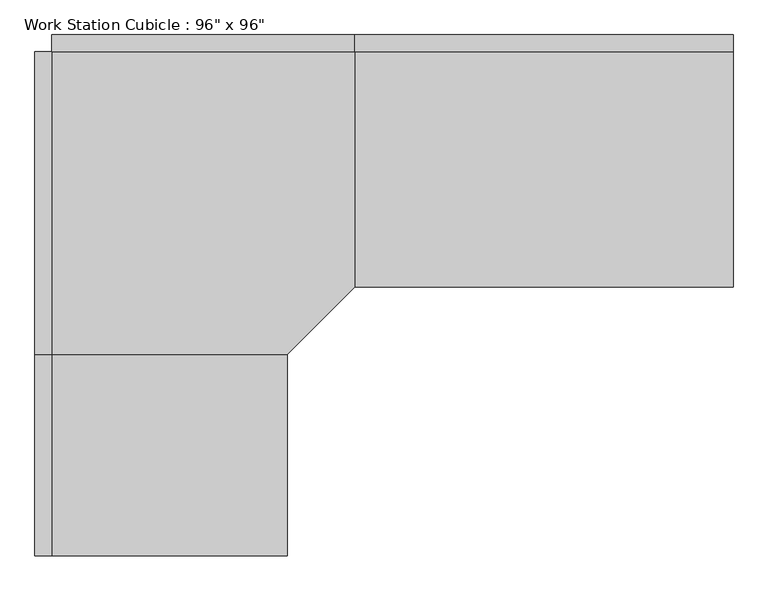
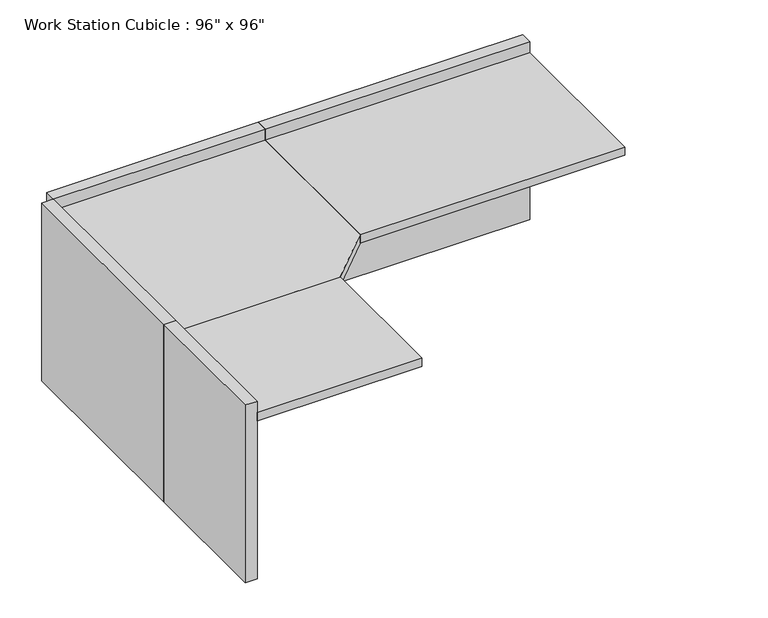
"""IFC4 building model written with IfcOpenShell, lengths in millimetres: furniture geometry."""

from ifc_helpers import new_model, si_unit, frame, origin, origin_with_axes, place, context, project, spatial, polyline, outline, extrude, source, transform, mapped, element, save


def furniture_e2d07697(model_context):
    return source(origin(), model_context, "Body", "SweptSolid", [
        extrude(outline(polyline([(-80.9317522, -545.8230076), (833.4682478, -545.8230076), (833.4682478, -1257.0230076), (630.2682478, -1460.2230076), (-80.9317522, -1460.2230076), (-80.9317522, -545.8230076)])), frame((0.0, 0.0, 723.9), z_axis=(0.0, 0.0, 1.0), x_axis=(1.0, 0.0, 0.0)), (0.0, 0.0, 1.0), 38.1),
        extrude(outline(polyline([(630.2682478, -2069.8230076), (-80.9317522, -2069.8230076), (-80.9317522, -1460.2230076), (630.2682478, -1460.2230076), (630.2682478, -2069.8230076)])), frame((0.0, 0.0, 723.9), z_axis=(0.0, 0.0, 1.0), x_axis=(1.0, 0.0, 0.0)), (0.0, 0.0, 1.0), 38.1),
        extrude(outline(polyline([(1976.4682478, -1257.0230076), (833.4682478, -1257.0230076), (833.4682478, -545.8230076), (1976.4682478, -545.8230076), (1976.4682478, -1257.0230076)])), frame((0.0, 0.0, 723.9), z_axis=(0.0, 0.0, 1.0), x_axis=(1.0, 0.0, 0.0)), (0.0, 0.0, 1.0), 38.1),
        extrude(outline(polyline([(1976.4682478, -545.8230076), (833.4682478, -545.8230076), (833.4682478, -495.0230076), (1976.4682478, -495.0230076), (1976.4682478, -545.8230076)])), origin_with_axes(), (0.0, 0.0, 1.0), 812.8),
        extrude(outline(polyline([(833.4682478, -545.8230076), (-80.9317522, -545.8230076), (-80.9317522, -495.0230076), (833.4682478, -495.0230076), (833.4682478, -545.8230076)])), origin_with_axes(), (0.0, 0.0, 1.0), 812.8),
        extrude(outline(polyline([(-80.9317522, -1460.2230076), (-131.7317522, -1460.2230076), (-131.7317522, -545.8230076), (-80.9317522, -545.8230076), (-80.9317522, -1460.2230076)])), origin_with_axes(), (0.0, 0.0, 1.0), 812.8),
        extrude(outline(polyline([(-80.9317522, -2069.8230076), (-131.7317522, -2069.8230076), (-131.7317522, -1460.2230076), (-80.9317522, -1460.2230076), (-80.9317522, -2069.8230076)])), origin_with_axes(), (0.0, 0.0, 1.0), 812.8),
    ])


if __name__ == "__main__":
    model = new_model("IFC4")
    model_context = context("Model", 3, world=origin())
    ifc_project = project(units=[si_unit("LENGTHUNIT", "METRE", prefix="MILLI")], contexts=[model_context])
    site = spatial("IfcSite", under=ifc_project)
    building = spatial("IfcBuilding", under=site)
    placement = place(None, origin())
    furniture_shape = furniture_e2d07697(model_context)
    element("IfcFurniture", 1, ObjectType="Work Station Cubicle : 96\" x 96\"", at=placement, inside=building, context=model_context, shape_type="MappedRepresentation", body=[
        mapped(furniture_shape, transform((0.0, 0.0, 0.0), x_axis=(1.0, 0.0, 0.0), y_axis=(0.0, 1.0, 0.0), z_axis=(0.0, 0.0, 1.0))),
    ])
    save(model, "model.ifc")

# Revit data of these elements
# Type "Work Station Cubicle : 96\" x 96\""
#   Assembly Code = "E2020"
#   Desktop Height = 2' - 6"
#   Desktop1 Width = 2' - 4"
#   Desktop2 Width = 2' - 4"
#   Panel Height = 2' - 8"
#   Panel1 Length = 2' - 0"
#   Panel2 Length = 3' - 9"
#   Cube Panel Material = Textile - Light Gray
#   Work Top Material = Laminate, Ivory, Matte
#   Default Elevation = 0
# Element 1 (IfcFurniture, "Work Station Cubicle : 96\" x 96\"")
#   Materials on its faces: "Textile - Light Gray", "Laminate, Ivory, Matte"
# Materials
#   "Textile - Light Gray": class "Fabric", colour RGB 204 204 204, transparency 0
#   "Laminate, Ivory, Matte": class "Plastic", colour RGB 247 247 239, transparency 0, Description = "Plastic Laminate - Ivory, Matte", Cost = 0
